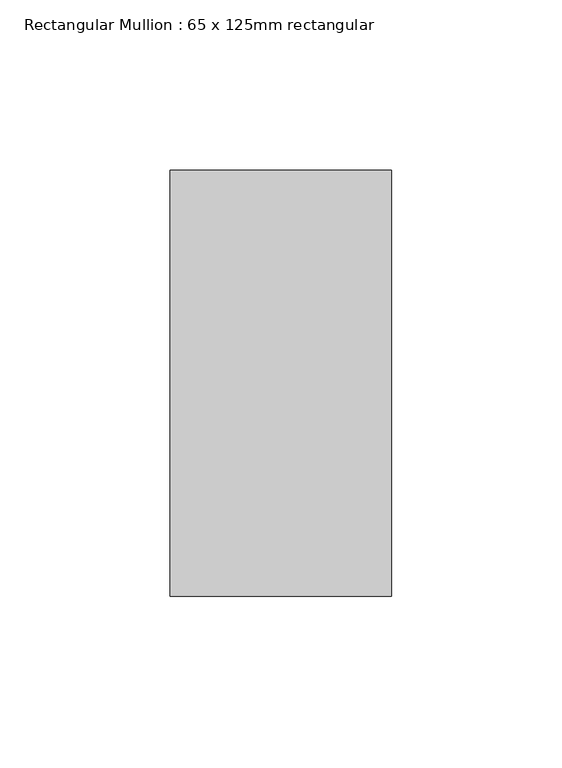
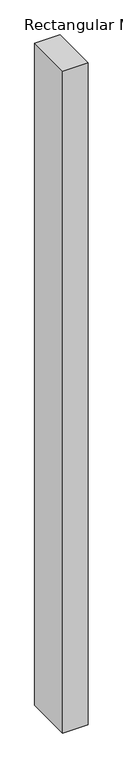
"""IFC4 building model written with IfcOpenShell, lengths in millimetres: member geometry, Rectangular Mullion : 65 x 125mm rectangular."""

from ifc_helpers import new_model, si_unit, frame, origin, place, context, project, spatial, polyline, outline, extrude, source, transform, mapped, element, save


def rectangular_mullion_65_x_125mm_rectangular_cb623ca7(model_context):
    return source(origin(), model_context, "Body", "SweptSolid", [
        extrude(outline(polyline([(0.0, 62.5), (0.0, -62.5), (-65.0, -62.5), (-65.0, 62.5), (0.0, 62.5)])), frame((0.0, 0.0, -1802.5), z_axis=(0.0, 0.0, 1.0), x_axis=(1.0, 0.0, 0.0)), (0.0, 0.0, 1.0), 1802.5),
    ])


if __name__ == "__main__":
    model = new_model("IFC4")
    model_context = context("Model", 3, world=origin())
    ifc_project = project(units=[si_unit("LENGTHUNIT", "METRE", prefix="MILLI")], contexts=[model_context])
    site = spatial("IfcSite", under=ifc_project)
    building = spatial("IfcBuilding", under=site)
    placement = place(None, origin())
    rectangular_mullion_65_x_125mm_rectangular_shape = rectangular_mullion_65_x_125mm_rectangular_cb623ca7(model_context)
    element("IfcMember", 1, ObjectType="Rectangular Mullion : 65 x 125mm rectangular", at=placement, inside=building, context=model_context, shape_type="MappedRepresentation", body=[
        mapped(rectangular_mullion_65_x_125mm_rectangular_shape, transform((0.0, 0.0, 0.0), x_axis=(1.0, 0.0, 0.0), y_axis=(0.0, 1.0, 0.0), z_axis=(0.0, 0.0, 1.0))),
    ])
    save(model, "model.ifc")

# Revit data of these elements
# Type "Rectangular Mullion : 65 x 125mm rectangular"
#   built-in parameter 1007304 = 0.410105 (stored number, unit not read)
#   built-in parameter 1007301 = 0.106627 (stored number, unit not read)
#   built-in parameter 1007300 = 0.106627 (stored number, unit not read)
# Element 1 (IfcMember, "Rectangular Mullion : 65 x 125mm rectangular")
#   Materials on its faces: "Aluminum"
# Materials
#   "Aluminum": class "Metal", colour RGB 244 245 246, transparency 0, Description = "Aluminum 6061", Cost = 0
